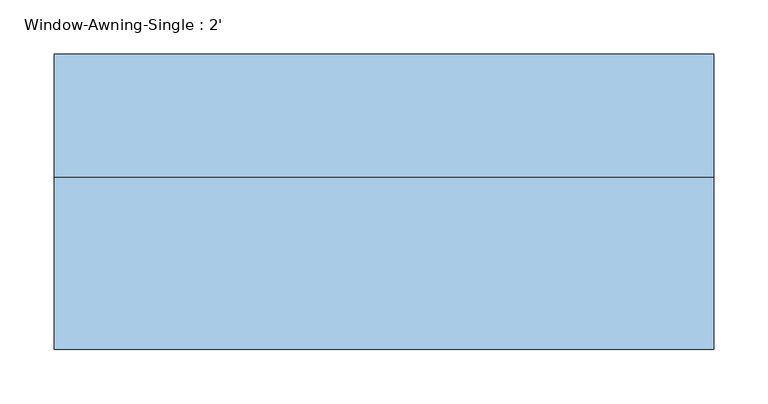
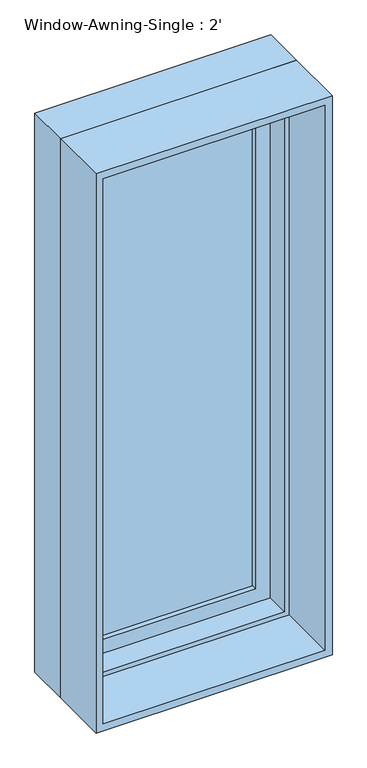
"""IFC4 building model written with IfcOpenShell, lengths in millimetres: window geometry, Window-Awning-Single : 2'."""

from ifc_helpers import new_model, si_unit, frame, origin, place, context, project, spatial, polyline, outline, extrude, faceted_brep, source, transform, mapped, element, save


def window_awning_single_2_9725ec62(model_context):
    return source(origin(), model_context, "Body", "SolidModel", [
        extrude(outline(polyline([(2438.4, -304.8), (914.4, -304.8), (914.4, 304.8), (2438.4, 304.8), (2438.4, -304.8)]), holes=[polyline([(2419.35, -285.75), (2419.35, 285.75), (933.45, 285.75), (933.45, -285.75), (2419.35, -285.75)])]), frame((0.0, -127.0, 0.0), z_axis=(0.0, 1.0, 0.0), x_axis=(0.0, 0.0, 1.0)), (0.0, 0.0, 1.0), 158.75),
        extrude(outline(polyline([(927.1, -292.1), (927.1, 292.1), (2425.7, 292.1), (2425.7, -292.1), (927.1, -292.1)]), holes=[polyline([(2368.55, -234.95), (2368.55, 234.95), (984.25, 234.95), (984.25, -234.95), (2368.55, -234.95)])]), frame((0.0, 95.25, 0.0), z_axis=(0.0, 1.0, 0.0), x_axis=(0.0, 0.0, 1.0)), (0.0, 0.0, 1.0), 44.45),
        extrude(outline(polyline([(234.95, 127.0), (234.95, 120.65), (-234.95, 120.65), (-234.95, 127.0), (234.95, 127.0)])), frame((0.0, 0.0, 984.25), z_axis=(0.0, 0.0, 1.0), x_axis=(1.0, 0.0, 0.0)), (0.0, 0.0, 1.0), 1384.3),
        extrude(outline(polyline([(234.95, 114.3), (234.95, 107.95), (-234.95, 107.95), (-234.95, 114.3), (234.95, 114.3)])), frame((0.0, 0.0, 984.25), z_axis=(0.0, 0.0, 1.0), x_axis=(1.0, 0.0, 0.0)), (0.0, 0.0, 1.0), 1384.3),
        faceted_brep([(292.1, 95.25, 927.1), (292.1, 146.05, 927.1), (-292.1, 146.05, 927.1), (-292.1, 95.25, 927.1), (273.05, 31.75, 946.15), (273.05, 95.25, 946.15), (-273.05, 95.25, 946.15), (-273.05, 31.75, 946.15), (304.8, 146.05, 914.4), (304.8, 31.75, 914.4), (-304.8, 31.75, 914.4), (-304.8, 146.05, 914.4), (-292.1, 146.05, 2425.7), (-292.1, 95.25, 2425.7), (-273.05, 95.25, 2406.65), (-273.05, 31.75, 2406.65), (-304.8, 31.75, 2438.4), (-304.8, 146.05, 2438.4), (292.1, 146.05, 2425.7), (292.1, 95.25, 2425.7), (273.05, 95.25, 2406.65), (273.05, 31.75, 2406.65), (304.8, 31.75, 2438.4), (304.8, 146.05, 2438.4)], [[[0, 1, 2, 3]], [[4, 5, 6, 7]], [[8, 9, 10, 11]], [[3, 2, 12, 13]], [[7, 6, 14, 15]], [[11, 10, 16, 17]], [[13, 12, 18, 19]], [[15, 14, 20, 21]], [[17, 16, 22, 23]], [[11, 17, 23, 8], [1, 18, 12, 2]], [[19, 18, 1, 0]], [[3, 13, 19, 0], [5, 20, 14, 6]], [[21, 20, 5, 4]], [[9, 22, 16, 10], [7, 15, 21, 4]], [[23, 22, 9, 8]]]),
    ])


if __name__ == "__main__":
    model = new_model("IFC4")
    model_context = context("Model", 3, world=origin())
    ifc_project = project(units=[si_unit("LENGTHUNIT", "METRE", prefix="MILLI")], contexts=[model_context])
    site = spatial("IfcSite", under=ifc_project)
    building = spatial("IfcBuilding", under=site)
    placement = place(None, origin())
    window_awning_single_2_shape = window_awning_single_2_9725ec62(model_context)
    element("IfcWindow", 1, ObjectType="Window-Awning-Single : 2'", at=placement, inside=building, context=model_context, shape_type="MappedRepresentation", body=[
        mapped(window_awning_single_2_shape, transform((0.0, 0.0, 0.0), x_axis=(1.0, 0.0, 0.0), y_axis=(0.0, 1.0, 0.0), z_axis=(0.0, 0.0, 1.0))),
    ])
    save(model, "model.ifc")

# Revit data of these elements
# Type "Window-Awning-Single : 2'"
#   Type Mark = "24"
#   Fire Rating = "0.5h"
#   Assembly Code = "B2020100"
#   Analytic Construction = "Double glazing - domestic"
#   Window Inset [instance default] = 0' - 0"
#   Wall Thickness [instance default] = 0' - 6"
#   Visual Light Transmittance = 0.81
#   Thermal Resistance (R) = 1.8146 (h·ft²·°F)/BTU
#   Solar Heat Gain Coefficient = 0.76
#   Rough Width = 2' - 0 1/2"
#   Rough Height = 5' - 0 1/2"
#   Interior Wall Closure [instance default] = 0' - 2 1/4"
#   Height = 5' - 0"
#   Heat Transfer Coefficient (U) = 0.5511 BTU/(h·ft²·°F)
#   Frame Extension [instance default] = 0' - 0 1/4"
#   Exterior Wall Closure [instance default] = 0' - 1 1/4"
#   Extension Jamb [instance default] = 0' - 2 1/4"
#   Default Sill Height = 3' - 0"
#   Width = 2' - 0"
#   Muntin Visibility = yes
#   Interior Trim Visibility [instance default] = yes
#   Exterior Trim Visibility [instance default] = yes
#   Extension Jamb Visibility [instance default] = yes
#   Muntin Pattern = Muntin Pattern_2x2 : Muntin Pattern_2x2
#   Interior Trim Material = Wood - Stained
#   Interior Trim = Trim-Window-Interior-Flat : Picture Frame
#   Interior Frame Material = Wood - Stained
#   Glass Panel Material = Glass
#   Exterior Trim Material = Clad - White
#   Exterior Trim = Trim-Window-Exterior-Flat : with Sill
#   Exterior Frame Material = Clad - White
#   Wall Closure = (empty or 0)
# Element 1 (IfcWindow, "Window-Awning-Single : 2'")
#   Wall Thickness = 0' - 10"
#   Extension Jamb = 0' - 6 1/4"
#   Materials on its faces: "Wood - Stained", "Glass", "Clad - White"
# Materials
#   "Wood - Stained": class "Wood", colour RGB 224 178 126, transparency 0, Cost = 0
#   "Glass": class "Glass", colour RGB 0 128 192, transparency 0.75, Description = "Soda Lime Glass", Cost = 0
#   "Clad - White": class "Wood", colour RGB 242 242 238, transparency 0, Cost = 0
